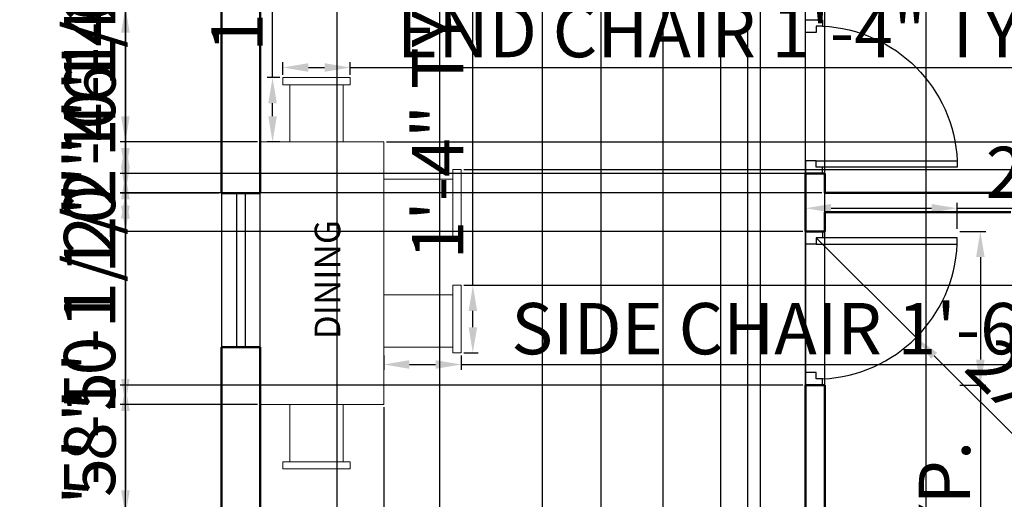
# Model space of a CAD drawing. Units: inches. Extents: x 1086 to 1501, y 383 to 973.
# Tile 3 of 7: x 1086 to 1316, y 611 to 723. Entities that reach past the tile are written whole.
import ezdxf

# ---------------------------------------------------------------- set-up
doc = ezdxf.new("R2010")
doc.units = ezdxf.units.IN
for name, color, linetype, lineweight in [('A-ANNO-DIMS', 2, 'Continuous', 18), ('A-AREA-IDEN', 7, 'Continuous', 25), ('door', 10, 'Continuous', 25), ('furniture', 255, 'Continuous', 18), ('wall', 7, 'Continuous', 50), ('window', 81, 'Continuous', 25)]:
    doc.layers.add(name, color=color, linetype=linetype, lineweight=lineweight)
doc.styles.get("Standard").update_dxf_attribs({"font": 'arial.ttf'})
doc.dimstyles.new('ISO-25', dxfattribs={"dimtxt": 12, "dimasz": 6, "dimexe": 1.25, "dimexo": 0.625, "dimtad": 1, "dimdec": 1, "dimlunit": 3, "dimtxsty": 'Standard', "dimcen": 2.5, "dimadec": 0, "dimazin": 0, "dimtfac": 1, "dimtdec": 1, "dimtmove": 0, "dimatfit": 3, "dimfxl": 1, "dimarcsym": 0})

# ---------------------------------------------------------------- blocks, each defined once
blk = doc.blocks.new('d2')
at = {"layer": 'door'}
blk.add_line((1603.89, 600.63), (1639.89, 600.63), dxfattribs=at)
blk.add_lwpolyline([(1605.39, 603.13), (1606.89, 603.13), (1606.89, 636.13), (1605.39, 636.13)], close=True, dxfattribs=at)
for points in [[(1606.89, 600.63), (1603.89, 600.63), (1603.89, 604.63), (1605.39, 604.63), (1605.39, 603.13), (1606.89, 603.13), (1606.89, 600.63)], [(1636.89, 600.63), (1639.89, 600.63), (1639.89, 604.63), (1638.39, 604.63), (1638.39, 603.13), (1636.89, 603.13), (1636.89, 600.63)]]:
    blk.add_lwpolyline(points, dxfattribs=at)
blk.add_arc((1605.39, 603.13), 33.03, 2.6026, 87.3974, dxfattribs=at)
blk = doc.blocks.new('w1')
at = {"layer": 'window'}
for p, q in [((1475.33, 845.32), (1475.33, 809.32)), ((1477.33, 845.32), (1477.33, 809.32))]:
    blk.add_line(p, q, dxfattribs=at)
blk.add_lwpolyline([(1471.83, 809.32), (1480.83, 809.32), (1480.83, 845.32), (1471.83, 845.32)], close=True, dxfattribs=at)
blk = doc.blocks.new('CHAIR-DINING-END')
for points in [[(0, 13.37), (15.81, 13.37), (15.81, 15.03), (0, 15.03)], [(1.64, 0), (14.11, 0), (14.11, 13.37), (1.64, 13.37)]]:
    blk.add_lwpolyline(points, close=True)
blk = doc.blocks.new('CHAIR-DINING-SIDE')
for points in [[(16.15, 15.81), (18.13, 15.81), (18.13, 0), (16.15, 0)], [(0, 13.58), (16.15, 13.58), (16.15, 1.34), (0, 1.34)]]:
    blk.add_lwpolyline(points, close=True)
blk = doc.blocks.new('*D19')
at = {"layer": 'A-ANNO-DIMS', "color": 0, "lineweight": -2, "transparency": 16777216}
for p, q in [((1306.05, 673.21), (1312.08, 673.21)), ((1310.83, 667.21), (1310.83, 643.21)), ((1306.05, 637.21), (1312.08, 637.21)), ((1310.83, 637.21), (1310.83, 411.12))]:
    blk.add_line(p, q, dxfattribs=at)
at = {"layer": 'A-ANNO-DIMS', "color": 0, "transparency": 16777216}
for points in [[(1309.83, 667.21), (1311.83, 667.21), (1310.83, 673.21)], [(1309.83, 643.21), (1311.83, 643.21), (1310.83, 637.21)]]:
    blk.add_solid(points, dxfattribs=at)
at = {"layer": 'Defpoints', "color": 0, "transparency": 16777216}
for p in [(1305.43, 673.21), (1305.43, 637.21), (1310.83, 637.21)]:
    blk.add_point(p, dxfattribs=at)
at = {"layer": 'A-ANNO-DIMS', "color": 0, "transparency": 16777216, "insert": (1303.99, 521.16), "char_height": 12, "attachment_point": 5, "rotation": 90}
blk.add_mtext('BEDROOM DOOR 3\'-0" TYP.', dxfattribs=at)
blk = doc.blocks.new('*D20')
at = {"layer": 'A-ANNO-DIMS', "color": 0, "lineweight": -2, "transparency": 16777216}
for p, q in [((1269.93, 673.83), (1269.93, 679.86)), ((1305.43, 673.83), (1305.43, 679.86)), ((1275.93, 678.61), (1299.43, 678.61)), ((1305.43, 678.61), (1423.32, 678.61))]:
    blk.add_line(p, q, dxfattribs=at)
at = {"layer": 'A-ANNO-DIMS', "color": 0, "transparency": 16777216}
for points in [[(1275.93, 679.61), (1275.93, 677.61), (1269.93, 678.61)], [(1299.43, 679.61), (1299.43, 677.61), (1305.43, 678.61)]]:
    blk.add_solid(points, dxfattribs=at)
at = {"layer": 'Defpoints', "color": 0, "transparency": 16777216}
for p in [(1305.43, 678.61), (1269.93, 673.21), (1305.43, 673.21)]:
    blk.add_point(p, dxfattribs=at)
at = {"layer": 'A-ANNO-DIMS', "color": 0, "transparency": 16777216, "insert": (1367.37, 685.44), "char_height": 12, "attachment_point": 5}
blk.add_mtext('2\'-11 1/2" TYP.', dxfattribs=at)
blk = doc.blocks.new('*D25')
at = {"layer": 'A-ANNO-DIMS', "color": 0, "lineweight": -2, "transparency": 16777216}
for p, q in [((1147.7, 709.78), (1147.7, 712.78)), ((1153.7, 711.53), (1157.51, 711.53)), ((1163.51, 709.78), (1163.51, 712.78)), ((1163.51, 711.53), (1340.15, 711.53))]:
    blk.add_line(p, q, dxfattribs=at)
at = {"layer": 'A-ANNO-DIMS', "color": 0, "transparency": 16777216}
for points in [[(1153.7, 712.53), (1153.7, 710.53), (1147.7, 711.53)], [(1157.51, 712.53), (1157.51, 710.53), (1163.51, 711.53)]]:
    blk.add_solid(points, dxfattribs=at)
at = {"layer": 'Defpoints', "color": 0, "transparency": 16777216}
for p in [(1163.51, 711.53), (1147.7, 709.16), (1163.51, 709.16)]:
    blk.add_point(p, dxfattribs=at)
at = {"layer": 'A-ANNO-DIMS', "color": 0, "transparency": 16777216, "insert": (1254.83, 718.36), "char_height": 12, "attachment_point": 5}
blk.add_mtext('END CHAIR 1\'-4" TYP.', dxfattribs=at)
blk = doc.blocks.new('*D26')
at = {"layer": 'A-ANNO-DIMS', "color": 0, "lineweight": -2, "transparency": 16777216}
for p, q in [((1145.33, 709.16), (1145.33, 788.42)), ((1147.07, 709.16), (1144.08, 709.16)), ((1145.33, 700.13), (1145.33, 703.16)), ((1147.07, 694.13), (1144.08, 694.13))]:
    blk.add_line(p, q, dxfattribs=at)
at = {"layer": 'A-ANNO-DIMS', "color": 0, "transparency": 16777216}
for points in [[(1144.33, 703.16), (1146.33, 703.16), (1145.33, 709.16)], [(1144.33, 700.13), (1146.33, 700.13), (1145.33, 694.13)]]:
    blk.add_solid(points, dxfattribs=at)
at = {"layer": 'Defpoints', "color": 0, "transparency": 16777216}
for p in [(1145.33, 709.16), (1147.7, 709.16), (1147.7, 694.13)]:
    blk.add_point(p, dxfattribs=at)
at = {"layer": 'A-ANNO-DIMS', "color": 0, "transparency": 16777216, "insert": (1138.57, 751.79), "char_height": 12, "attachment_point": 5, "rotation": 90}
blk.add_mtext('1\'-3" TYP.', dxfattribs=at)
blk = doc.blocks.new('*D27')
at = {"layer": 'A-ANNO-DIMS', "color": 0, "lineweight": -2, "transparency": 16777216}
for p, q in [((1171.32, 644.17), (1171.32, 640.82)), ((1189.45, 644.17), (1189.45, 640.82)), ((1177.32, 642.07), (1183.45, 642.07)), ((1189.45, 642.07), (1370.39, 642.07))]:
    blk.add_line(p, q, dxfattribs=at)
at = {"layer": 'A-ANNO-DIMS', "color": 0, "transparency": 16777216}
for points in [[(1177.32, 643.07), (1177.32, 641.07), (1171.32, 642.07)], [(1183.45, 643.07), (1183.45, 641.07), (1189.45, 642.07)]]:
    blk.add_solid(points, dxfattribs=at)
at = {"layer": 'Defpoints', "color": 0, "transparency": 16777216}
for p in [(1171.32, 644.79), (1189.45, 644.79), (1189.45, 642.07)]:
    blk.add_point(p, dxfattribs=at)
at = {"layer": 'A-ANNO-DIMS', "color": 0, "transparency": 16777216, "insert": (1282.92, 648.9), "char_height": 12, "attachment_point": 5}
blk.add_mtext('SIDE CHAIR 1\'-6" TYP.', dxfattribs=at)
blk = doc.blocks.new('*D28')
at = {"layer": 'A-ANNO-DIMS', "color": 0, "lineweight": -2, "transparency": 16777216}
for p, q in [((1192.17, 660.6), (1192.17, 739.87)), ((1190.08, 660.6), (1193.42, 660.6)), ((1192.17, 650.79), (1192.17, 654.6)), ((1190.08, 644.79), (1193.42, 644.79))]:
    blk.add_line(p, q, dxfattribs=at)
at = {"layer": 'A-ANNO-DIMS', "color": 0, "transparency": 16777216}
for points in [[(1191.17, 654.6), (1193.17, 654.6), (1192.17, 660.6)], [(1191.17, 650.79), (1193.17, 650.79), (1192.17, 644.79)]]:
    blk.add_solid(points, dxfattribs=at)
at = {"layer": 'Defpoints', "color": 0, "transparency": 16777216}
for p in [(1189.45, 660.6), (1192.17, 660.6), (1189.45, 644.79)]:
    blk.add_point(p, dxfattribs=at)
at = {"layer": 'A-ANNO-DIMS', "color": 0, "transparency": 16777216, "insert": (1185.52, 703.24), "char_height": 12, "attachment_point": 5, "rotation": 90}
blk.add_mtext('1\'-4" TYP.', dxfattribs=at)
blk = doc.blocks.new('*D33')
at = {"layer": 'A-ANNO-DIMS', "color": 0, "lineweight": -2, "transparency": 16777216}
for p, q in [((1132.8, 760.21), (1109.68, 760.21)), ((1110.93, 754.21), (1110.93, 688.12)), ((1132.8, 682.12), (1109.68, 682.12))]:
    blk.add_line(p, q, dxfattribs=at)
at = {"layer": 'A-ANNO-DIMS', "color": 0, "transparency": 16777216}
for points in [[(1109.93, 754.21), (1111.93, 754.21), (1110.93, 760.21)], [(1109.93, 688.12), (1111.93, 688.12), (1110.93, 682.12)]]:
    blk.add_solid(points, dxfattribs=at)
at = {"layer": 'Defpoints', "color": 0, "transparency": 16777216}
for p in [(1133.43, 760.21), (1110.93, 682.12), (1133.43, 682.12)]:
    blk.add_point(p, dxfattribs=at)
at = {"layer": 'A-ANNO-DIMS', "color": 0, "transparency": 16777216, "insert": (1104.18, 721.16), "char_height": 12, "attachment_point": 5, "rotation": 90}
blk.add_mtext('6\'-6"', dxfattribs=at)
blk = doc.blocks.new('*D40')
at = {"layer": 'A-ANNO-DIMS', "color": 0, "lineweight": -2, "transparency": 16777216}
for p, q in [((1142.43, 502.33), (1142.43, 867.19)), ((1148.43, 865.94), (1263.93, 865.94)), ((1269.93, 502.33), (1269.93, 867.19))]:
    blk.add_line(p, q, dxfattribs=at)
at = {"layer": 'A-ANNO-DIMS', "color": 0, "transparency": 16777216}
for points in [[(1148.43, 866.94), (1148.43, 864.94), (1142.43, 865.94)], [(1263.93, 866.94), (1263.93, 864.94), (1269.93, 865.94)]]:
    blk.add_solid(points, dxfattribs=at)
at = {"layer": 'Defpoints', "color": 0, "transparency": 16777216}
for p in [(1269.93, 865.94), (1142.43, 501.71), (1269.93, 501.71)]:
    blk.add_point(p, dxfattribs=at)
at = {"layer": 'A-ANNO-DIMS', "color": 0, "transparency": 16777216, "insert": (1206.18, 872.77), "char_height": 12, "attachment_point": 5}
blk.add_mtext('10\'-7 1/2"', dxfattribs=at)
blk = doc.blocks.new('*D41')
at = {"layer": 'A-ANNO-DIMS', "color": 0, "lineweight": -2, "transparency": 16777216}
for p, q in [((1141.8, 725.71), (1109.68, 725.71)), ((1110.93, 507.71), (1110.93, 719.71)), ((1141.8, 501.71), (1109.68, 501.71))]:
    blk.add_line(p, q, dxfattribs=at)
at = {"layer": 'A-ANNO-DIMS', "color": 0, "transparency": 16777216}
for points in [[(1109.93, 719.71), (1111.93, 719.71), (1110.93, 725.71)], [(1109.93, 507.71), (1111.93, 507.71), (1110.93, 501.71)]]:
    blk.add_solid(points, dxfattribs=at)
at = {"layer": 'Defpoints', "color": 0, "transparency": 16777216}
for p in [(1110.93, 725.71), (1142.43, 725.71), (1142.43, 501.71)]:
    blk.add_point(p, dxfattribs=at)
at = {"layer": 'A-ANNO-DIMS', "color": 0, "transparency": 16777216, "insert": (1104.18, 613.71), "char_height": 12, "attachment_point": 5, "rotation": 90}
blk.add_mtext('18\'-8"', dxfattribs=at)
blk = doc.blocks.new('*D42')
at = {"layer": 'A-ANNO-DIMS', "color": 0, "lineweight": -2, "transparency": 16777216}
for p, q in [((1256.43, 502.33), (1256.43, 867.19)), ((1262.43, 865.94), (1263.93, 865.94)), ((1269.93, 502.33), (1269.93, 867.19)), ((1269.93, 865.94), (1335.91, 865.94))]:
    blk.add_line(p, q, dxfattribs=at)
at = {"layer": 'A-ANNO-DIMS', "color": 0, "transparency": 16777216}
for points in [[(1262.43, 866.94), (1262.43, 864.94), (1256.43, 865.94)], [(1263.93, 866.94), (1263.93, 864.94), (1269.93, 865.94)]]:
    blk.add_solid(points, dxfattribs=at)
at = {"layer": 'Defpoints', "color": 0, "transparency": 16777216}
for p in [(1269.93, 865.94), (1256.43, 501.71), (1269.93, 501.71)]:
    blk.add_point(p, dxfattribs=at)
at = {"layer": 'A-ANNO-DIMS', "color": 0, "transparency": 16777216, "insert": (1305.92, 872.77), "char_height": 12, "attachment_point": 5}
blk.add_mtext('1\'-1 1/2"', dxfattribs=at)
blk = doc.blocks.new('*D43')
at = {"layer": 'A-ANNO-DIMS', "color": 0, "lineweight": -2, "transparency": 16777216}
for p, q in [((1208.43, 497.83), (1208.43, 867.19)), ((1214.43, 865.94), (1250.43, 865.94)), ((1256.43, 497.83), (1256.43, 867.19))]:
    blk.add_line(p, q, dxfattribs=at)
at = {"layer": 'A-ANNO-DIMS', "color": 0, "transparency": 16777216}
for points in [[(1214.43, 866.94), (1214.43, 864.94), (1208.43, 865.94)], [(1250.43, 866.94), (1250.43, 864.94), (1256.43, 865.94)]]:
    blk.add_solid(points, dxfattribs=at)
at = {"layer": 'Defpoints', "color": 0, "transparency": 16777216}
for p in [(1256.43, 865.94), (1208.43, 497.21), (1256.43, 497.21)]:
    blk.add_point(p, dxfattribs=at)
at = {"layer": 'A-ANNO-DIMS', "color": 0, "transparency": 16777216, "insert": (1232.43, 872.69), "char_height": 12, "attachment_point": 5}
blk.add_mtext('4\'-0"', dxfattribs=at)
blk = doc.blocks.new('*D45')
at = {"layer": 'A-ANNO-DIMS', "color": 0, "lineweight": -2, "transparency": 16777216}
for p, q in [((1259.43, 497.83), (1259.43, 867.19)), ((1265.43, 865.94), (1352.43, 865.94)), ((1358.43, 497.83), (1358.43, 867.19))]:
    blk.add_line(p, q, dxfattribs=at)
at = {"layer": 'A-ANNO-DIMS', "color": 0, "transparency": 16777216}
for points in [[(1265.43, 866.94), (1265.43, 864.94), (1259.43, 865.94)], [(1352.43, 866.94), (1352.43, 864.94), (1358.43, 865.94)]]:
    blk.add_solid(points, dxfattribs=at)
at = {"layer": 'Defpoints', "color": 0, "transparency": 16777216}
for p in [(1358.43, 865.94), (1259.43, 497.21), (1358.43, 497.21)]:
    blk.add_point(p, dxfattribs=at)
at = {"layer": 'A-ANNO-DIMS', "color": 0, "transparency": 16777216, "insert": (1308.93, 872.7), "char_height": 12, "attachment_point": 5}
blk.add_mtext('8\'-3"', dxfattribs=at)
blk = doc.blocks.new('*D49')
at = {"layer": 'A-ANNO-DIMS', "color": 0, "lineweight": -2, "transparency": 16777216}
for p, q in [((1110.93, 760.21), (1110.93, 766.21)), ((1218.3, 754.21), (1109.68, 754.21)), ((1110.93, 754.21), (1110.93, 749.71)), ((1218.3, 749.71), (1109.68, 749.71)), ((1110.93, 743.71), (1110.93, 676.6))]:
    blk.add_line(p, q, dxfattribs=at)
at = {"layer": 'A-ANNO-DIMS', "color": 0, "transparency": 16777216}
for points in [[(1109.93, 760.21), (1111.93, 760.21), (1110.93, 754.21)], [(1109.93, 743.71), (1111.93, 743.71), (1110.93, 749.71)]]:
    blk.add_solid(points, dxfattribs=at)
at = {"layer": 'Defpoints', "color": 0, "transparency": 16777216}
for p in [(1218.93, 754.21), (1110.93, 749.71), (1218.93, 749.71)]:
    blk.add_point(p, dxfattribs=at)
at = {"layer": 'A-ANNO-DIMS', "color": 0, "transparency": 16777216, "insert": (1104.1, 707.15), "char_height": 12, "attachment_point": 5, "rotation": 90}
blk.add_mtext('0\'-4 1/2"', dxfattribs=at)
blk = doc.blocks.new('*D50')
at = {"layer": 'A-ANNO-DIMS', "color": 0, "lineweight": -2, "transparency": 16777216}
for p, q in [((1184.43, 502.33), (1184.43, 867.19)), ((1190.43, 865.94), (1202.43, 865.94)), ((1208.43, 502.33), (1208.43, 867.19)), ((1208.43, 865.94), (1247.78, 865.94))]:
    blk.add_line(p, q, dxfattribs=at)
at = {"layer": 'A-ANNO-DIMS', "color": 0, "transparency": 16777216}
for points in [[(1190.43, 866.94), (1190.43, 864.94), (1184.43, 865.94)], [(1202.43, 866.94), (1202.43, 864.94), (1208.43, 865.94)]]:
    blk.add_solid(points, dxfattribs=at)
at = {"layer": 'Defpoints', "color": 0, "transparency": 16777216}
for p in [(1208.43, 865.94), (1184.43, 501.71), (1208.43, 501.71)]:
    blk.add_point(p, dxfattribs=at)
at = {"layer": 'A-ANNO-DIMS', "color": 0, "transparency": 16777216, "insert": (1231.11, 872.69), "char_height": 12, "attachment_point": 5}
blk.add_mtext('2\'-0"', dxfattribs=at)
blk = doc.blocks.new('*D52')
at = {"layer": 'A-ANNO-DIMS', "color": 0, "lineweight": -2, "transparency": 16777216}
for p, q in [((1110.93, 692.71), (1110.93, 759.82)), ((1273.8, 686.71), (1109.68, 686.71)), ((1110.93, 682.21), (1110.93, 686.71)), ((1273.8, 682.21), (1109.68, 682.21)), ((1110.93, 676.21), (1110.93, 670.21))]:
    blk.add_line(p, q, dxfattribs=at)
at = {"layer": 'A-ANNO-DIMS', "color": 0, "transparency": 16777216}
for points in [[(1109.93, 692.71), (1111.93, 692.71), (1110.93, 686.71)], [(1109.93, 676.21), (1111.93, 676.21), (1110.93, 682.21)]]:
    blk.add_solid(points, dxfattribs=at)
at = {"layer": 'Defpoints', "color": 0, "transparency": 16777216}
for p in [(1110.93, 686.71), (1274.43, 686.71), (1274.43, 682.21)]:
    blk.add_point(p, dxfattribs=at)
at = {"layer": 'A-ANNO-DIMS', "color": 0, "transparency": 16777216, "insert": (1104.1, 729.26), "char_height": 12, "attachment_point": 5, "rotation": 90}
blk.add_mtext('0\'-4 1/2"', dxfattribs=at)
blk = doc.blocks.new('*D53')
at = {"layer": 'A-ANNO-DIMS', "color": 0, "lineweight": -2, "transparency": 16777216}
for p, q in [((1110.93, 686.71), (1110.93, 752.69)), ((1269.3, 686.71), (1109.68, 686.71)), ((1110.93, 679.21), (1110.93, 680.71)), ((1269.3, 673.21), (1109.68, 673.21))]:
    blk.add_line(p, q, dxfattribs=at)
at = {"layer": 'A-ANNO-DIMS', "color": 0, "transparency": 16777216}
for points in [[(1109.93, 680.71), (1111.93, 680.71), (1110.93, 686.71)], [(1109.93, 679.21), (1111.93, 679.21), (1110.93, 673.21)]]:
    blk.add_solid(points, dxfattribs=at)
at = {"layer": 'Defpoints', "color": 0, "transparency": 16777216}
for p in [(1110.93, 686.71), (1269.93, 686.71), (1269.93, 673.21)]:
    blk.add_point(p, dxfattribs=at)
at = {"layer": 'A-ANNO-DIMS', "color": 0, "transparency": 16777216, "insert": (1104.1, 722.7), "char_height": 12, "attachment_point": 5, "rotation": 90}
blk.add_mtext('1\'-1 1/2"', dxfattribs=at)
blk = doc.blocks.new('*D58')
at = {"layer": 'A-ANNO-DIMS', "color": 0, "lineweight": -2, "transparency": 16777216}
for p, q in [((1250.08, 809.82), (1250.08, 392.46)), ((1222.08, 799.32), (1222.08, 392.46)), ((1228.08, 393.71), (1244.08, 393.71)), ((1250.08, 393.71), (1289.44, 393.71))]:
    blk.add_line(p, q, dxfattribs=at)
at = {"layer": 'A-ANNO-DIMS', "color": 0, "transparency": 16777216}
for points in [[(1228.08, 394.71), (1228.08, 392.71), (1222.08, 393.71)], [(1244.08, 394.71), (1244.08, 392.71), (1250.08, 393.71)]]:
    blk.add_solid(points, dxfattribs=at)
at = {"layer": 'Defpoints', "color": 0, "transparency": 16777216}
for p in [(1250.08, 810.44), (1222.08, 799.94), (1250.08, 393.71)]:
    blk.add_point(p, dxfattribs=at)
at = {"layer": 'A-ANNO-DIMS', "color": 0, "transparency": 16777216, "insert": (1272.76, 400.36), "char_height": 12, "attachment_point": 5}
blk.add_mtext('2\'-4"', dxfattribs=at)
blk = doc.blocks.new('*D60')
at = {"layer": 'A-ANNO-DIMS', "color": 0, "lineweight": -2, "transparency": 16777216}
for p, q in [((1322.43, 629.08), (1322.43, 392.46)), ((1326.93, 629.08), (1326.93, 392.46)), ((1316.43, 393.71), (1310.43, 393.71)), ((1322.43, 393.71), (1326.93, 393.71)), ((1332.93, 393.71), (1400.04, 393.71))]:
    blk.add_line(p, q, dxfattribs=at)
at = {"layer": 'A-ANNO-DIMS', "color": 0, "transparency": 16777216}
for points in [[(1316.43, 394.71), (1316.43, 392.71), (1322.43, 393.71)], [(1332.93, 394.71), (1332.93, 392.71), (1326.93, 393.71)]]:
    blk.add_solid(points, dxfattribs=at)
at = {"layer": 'Defpoints', "color": 0, "transparency": 16777216}
for p in [(1322.43, 629.71), (1326.93, 629.71), (1326.93, 393.71)]:
    blk.add_point(p, dxfattribs=at)
at = {"layer": 'A-ANNO-DIMS', "color": 0, "transparency": 16777216, "insert": (1369.49, 400.54), "char_height": 12, "attachment_point": 5}
blk.add_mtext('0\'-4 1/2"', dxfattribs=at)
blk = doc.blocks.new('*D61')
at = {"layer": 'A-ANNO-DIMS', "color": 0, "lineweight": -2, "transparency": 16777216}
for p, q in [((1376.11, 865.94), (1310.13, 865.94)), ((1382.11, 674.69), (1382.11, 867.19)), ((1394.43, 865.94), (1382.11, 865.94)), ((1394.43, 678.33), (1394.43, 867.19)), ((1400.43, 865.94), (1406.43, 865.94))]:
    blk.add_line(p, q, dxfattribs=at)
at = {"layer": 'A-ANNO-DIMS', "color": 0, "transparency": 16777216}
for points in [[(1376.11, 866.94), (1376.11, 864.94), (1382.11, 865.94)], [(1400.43, 866.94), (1400.43, 864.94), (1394.43, 865.94)]]:
    blk.add_solid(points, dxfattribs=at)
at = {"layer": 'Defpoints', "color": 0, "transparency": 16777216}
for p in [(1382.11, 865.94), (1394.43, 677.71), (1382.11, 674.06)]:
    blk.add_point(p, dxfattribs=at)
at = {"layer": 'A-ANNO-DIMS', "color": 0, "transparency": 16777216, "insert": (1340.12, 872.77), "char_height": 12, "attachment_point": 5}
blk.add_mtext('1\'-0 1/2"', dxfattribs=at)
blk = doc.blocks.new('*D63')
at = {"layer": 'A-ANNO-DIMS', "color": 0, "lineweight": -2, "transparency": 16777216}
for p, q in [((1142.43, 632.08), (1142.43, 392.46)), ((1171.32, 632.08), (1171.32, 392.46)), ((1148.43, 393.71), (1165.32, 393.71)), ((1171.32, 393.71), (1210.68, 393.71))]:
    blk.add_line(p, q, dxfattribs=at)
at = {"layer": 'A-ANNO-DIMS', "color": 0, "transparency": 16777216}
for points in [[(1148.43, 394.71), (1148.43, 392.71), (1142.43, 393.71)], [(1165.32, 394.71), (1165.32, 392.71), (1171.32, 393.71)]]:
    blk.add_solid(points, dxfattribs=at)
at = {"layer": 'Defpoints', "color": 0, "transparency": 16777216}
for p in [(1142.43, 632.71), (1171.32, 632.71), (1171.32, 393.71)]:
    blk.add_point(p, dxfattribs=at)
at = {"layer": 'A-ANNO-DIMS', "color": 0, "transparency": 16777216, "insert": (1194, 400.46), "char_height": 12, "attachment_point": 5}
blk.add_mtext('2\'-5"', dxfattribs=at)
blk = doc.blocks.new('*D64')
at = {"layer": 'A-ANNO-DIMS', "color": 0, "lineweight": -2, "transparency": 16777216}
for p, q in [((1141.8, 694.13), (1109.68, 694.13)), ((1110.93, 688.13), (1110.93, 638.71)), ((1141.8, 632.71), (1109.68, 632.71))]:
    blk.add_line(p, q, dxfattribs=at)
at = {"layer": 'A-ANNO-DIMS', "color": 0, "transparency": 16777216}
for points in [[(1109.93, 688.13), (1111.93, 688.13), (1110.93, 694.13)], [(1109.93, 638.71), (1111.93, 638.71), (1110.93, 632.71)]]:
    blk.add_solid(points, dxfattribs=at)
at = {"layer": 'Defpoints', "color": 0, "transparency": 16777216}
for p in [(1142.43, 694.13), (1110.93, 632.71), (1142.43, 632.71)]:
    blk.add_point(p, dxfattribs=at)
at = {"layer": 'A-ANNO-DIMS', "color": 0, "transparency": 16777216, "insert": (1104.1, 663.42), "char_height": 12, "attachment_point": 5, "rotation": 90}
blk.add_mtext('5\'-1 1/2"', dxfattribs=at)
blk = doc.blocks.new('*D65')
at = {"layer": 'A-ANNO-DIMS', "color": 0, "lineweight": -2, "transparency": 16777216}
for p, q in [((1110.93, 725.71), (1110.93, 793.02)), ((1141.8, 725.71), (1109.68, 725.71)), ((1110.93, 700.13), (1110.93, 719.71)), ((1141.8, 694.13), (1109.68, 694.13))]:
    blk.add_line(p, q, dxfattribs=at)
at = {"layer": 'A-ANNO-DIMS', "color": 0, "transparency": 16777216}
for points in [[(1109.93, 719.71), (1111.93, 719.71), (1110.93, 725.71)], [(1109.93, 700.13), (1111.93, 700.13), (1110.93, 694.13)]]:
    blk.add_solid(points, dxfattribs=at)
at = {"layer": 'Defpoints', "color": 0, "transparency": 16777216}
for p in [(1110.93, 725.71), (1142.43, 725.71), (1142.43, 694.13)]:
    blk.add_point(p, dxfattribs=at)
at = {"layer": 'A-ANNO-DIMS', "color": 0, "transparency": 16777216, "insert": (1104.1, 762.36), "char_height": 12, "attachment_point": 5, "rotation": 90}
blk.add_mtext('2\'-7 1/2"', dxfattribs=at)
blk = doc.blocks.new('*D66')
at = {"layer": 'A-ANNO-DIMS', "color": 0, "lineweight": -2, "transparency": 16777216}
for p, q in [((1190.08, 687.66), (1428.36, 687.66)), ((1427.11, 681.66), (1427.11, 666.6)), ((1190.08, 660.6), (1428.36, 660.6)), ((1427.11, 660.6), (1427.11, 621.25))]:
    blk.add_line(p, q, dxfattribs=at)
at = {"layer": 'A-ANNO-DIMS', "color": 0, "transparency": 16777216}
for points in [[(1426.11, 681.66), (1428.11, 681.66), (1427.11, 687.66)], [(1426.11, 666.6), (1428.11, 666.6), (1427.11, 660.6)]]:
    blk.add_solid(points, dxfattribs=at)
at = {"layer": 'Defpoints', "color": 0, "transparency": 16777216}
for p in [(1189.45, 687.66), (1189.45, 660.6), (1427.11, 660.6)]:
    blk.add_point(p, dxfattribs=at)
at = {"layer": 'A-ANNO-DIMS', "color": 0, "transparency": 16777216, "insert": (1420.36, 637.93), "char_height": 12, "attachment_point": 5, "rotation": 90}
blk.add_mtext('2\'-3"', dxfattribs=at)
blk = doc.blocks.new('*D67')
at = {"layer": 'A-ANNO-DIMS', "color": 0, "lineweight": -2, "transparency": 16777216}
for p, q in [((1427.11, 700.13), (1427.11, 706.13)), ((1171.95, 694.13), (1428.36, 694.13)), ((1427.11, 694.13), (1427.11, 687.66)), ((1190.08, 687.66), (1428.36, 687.66)), ((1427.11, 681.66), (1427.11, 614.55))]:
    blk.add_line(p, q, dxfattribs=at)
at = {"layer": 'A-ANNO-DIMS', "color": 0, "transparency": 16777216}
for points in [[(1426.11, 700.13), (1428.11, 700.13), (1427.11, 694.13)], [(1426.11, 681.66), (1428.11, 681.66), (1427.11, 687.66)]]:
    blk.add_solid(points, dxfattribs=at)
at = {"layer": 'Defpoints', "color": 0, "transparency": 16777216}
for p in [(1171.32, 694.13), (1189.45, 687.66), (1427.11, 687.66)]:
    blk.add_point(p, dxfattribs=at)
at = {"layer": 'A-ANNO-DIMS', "color": 0, "transparency": 16777216, "insert": (1420.28, 645.1), "char_height": 12, "attachment_point": 5, "rotation": 90}
blk.add_mtext('0\'-6 1/2"', dxfattribs=at)
blk = doc.blocks.new('*D68')
at = {"layer": 'A-ANNO-DIMS', "color": 0, "lineweight": -2, "transparency": 16777216}
for p, q in [((1110.93, 606.65), (1110.93, 683.08)), ((1262.93, 606.65), (1109.68, 606.65)), ((1110.93, 542.31), (1110.93, 600.65)), ((1262.93, 536.31), (1109.68, 536.31))]:
    blk.add_line(p, q, dxfattribs=at)
at = {"layer": 'A-ANNO-DIMS', "color": 0, "transparency": 16777216}
for points in [[(1109.93, 600.65), (1111.93, 600.65), (1110.93, 606.65)], [(1109.93, 542.31), (1111.93, 542.31), (1110.93, 536.31)]]:
    blk.add_solid(points, dxfattribs=at)
at = {"layer": 'Defpoints', "color": 0, "transparency": 16777216}
for p in [(1110.93, 606.65), (1263.55, 606.65), (1263.55, 536.31)]:
    blk.add_point(p, dxfattribs=at)
at = {"layer": 'A-ANNO-DIMS', "color": 0, "transparency": 16777216, "insert": (1104.1, 647.86), "char_height": 12, "attachment_point": 5, "rotation": 90}
blk.add_mtext('5\'-10 1/2"', dxfattribs=at)
blk = doc.blocks.new('*D69')
at = {"layer": 'A-ANNO-DIMS', "color": 0, "lineweight": -2, "transparency": 16777216}
for p, q in [((1236.63, 603.21), (1236.63, 867.19)), ((1242.63, 865.94), (1263.93, 865.94)), ((1269.93, 603.25), (1269.93, 867.19)), ((1269.93, 865.94), (1337.25, 865.94))]:
    blk.add_line(p, q, dxfattribs=at)
at = {"layer": 'A-ANNO-DIMS', "color": 0, "transparency": 16777216}
for points in [[(1242.63, 866.94), (1242.63, 864.94), (1236.63, 865.94)], [(1263.93, 866.94), (1263.93, 864.94), (1269.93, 865.94)]]:
    blk.add_solid(points, dxfattribs=at)
at = {"layer": 'Defpoints', "color": 0, "transparency": 16777216}
for p in [(1269.93, 865.94), (1236.63, 602.59), (1269.93, 602.62)]:
    blk.add_point(p, dxfattribs=at)
at = {"layer": 'A-ANNO-DIMS', "color": 0, "transparency": 16777216, "insert": (1306.59, 872.77), "char_height": 12, "attachment_point": 5}
blk.add_mtext('2\'-9 1/2"', dxfattribs=at)
blk = doc.blocks.new('*D70')
at = {"layer": 'A-ANNO-DIMS', "color": 0, "lineweight": -2, "transparency": 16777216}
for p, q in [((1269.3, 637.21), (1109.68, 637.21)), ((1110.93, 631.21), (1110.93, 612.65)), ((1262.93, 606.65), (1109.68, 606.65)), ((1110.93, 606.65), (1110.93, 539.33))]:
    blk.add_line(p, q, dxfattribs=at)
at = {"layer": 'A-ANNO-DIMS', "color": 0, "transparency": 16777216}
for points in [[(1109.93, 631.21), (1111.93, 631.21), (1110.93, 637.21)], [(1109.93, 612.65), (1111.93, 612.65), (1110.93, 606.65)]]:
    blk.add_solid(points, dxfattribs=at)
at = {"layer": 'Defpoints', "color": 0, "transparency": 16777216}
for p in [(1269.93, 637.21), (1110.93, 606.65), (1263.55, 606.65)]:
    blk.add_point(p, dxfattribs=at)
at = {"layer": 'A-ANNO-DIMS', "color": 0, "transparency": 16777216, "insert": (1104.1, 569.99), "char_height": 12, "attachment_point": 5, "rotation": 90}
blk.add_mtext('2\'-6 1/2"', dxfattribs=at)
blk = doc.blocks.new('*D71')
at = {"layer": 'A-ANNO-DIMS', "color": 0, "lineweight": -2, "transparency": 16777216}
for p, q in [((1142.43, 589.29), (1142.43, 867.19)), ((1148.43, 865.94), (1154.43, 865.94)), ((1160.43, 589.29), (1160.43, 867.19)), ((1160.43, 865.94), (1198.45, 865.94))]:
    blk.add_line(p, q, dxfattribs=at)
at = {"layer": 'A-ANNO-DIMS', "color": 0, "transparency": 16777216}
for points in [[(1148.43, 866.94), (1148.43, 864.94), (1142.43, 865.94)], [(1154.43, 866.94), (1154.43, 864.94), (1160.43, 865.94)]]:
    blk.add_solid(points, dxfattribs=at)
at = {"layer": 'Defpoints', "color": 0, "transparency": 16777216}
for p in [(1160.43, 865.94), (1142.43, 588.67), (1160.43, 588.67)]:
    blk.add_point(p, dxfattribs=at)
at = {"layer": 'A-ANNO-DIMS', "color": 0, "transparency": 16777216, "insert": (1182.44, 872.69), "char_height": 12, "attachment_point": 5}
blk.add_mtext('1\'-6"', dxfattribs=at)
blk = doc.blocks.new('*D75')
at = {"layer": 'A-ANNO-DIMS', "color": 0, "lineweight": -2, "transparency": 16777216}
for p, q in [((1274.43, 723.33), (1274.43, 867.19)), ((1280.43, 865.94), (1304.55, 865.94)), ((1310.55, 724.51), (1310.55, 867.19))]:
    blk.add_line(p, q, dxfattribs=at)
at = {"layer": 'A-ANNO-DIMS', "color": 0, "transparency": 16777216}
for points in [[(1280.43, 866.94), (1280.43, 864.94), (1274.43, 865.94)], [(1304.55, 866.94), (1304.55, 864.94), (1310.55, 865.94)]]:
    blk.add_solid(points, dxfattribs=at)
at = {"layer": 'Defpoints', "color": 0, "transparency": 16777216}
for p in [(1310.55, 865.94), (1310.55, 723.89), (1274.43, 722.71)]:
    blk.add_point(p, dxfattribs=at)
at = {"layer": 'A-ANNO-DIMS', "color": 0, "transparency": 16777216, "insert": (1292.49, 872.7), "char_height": 12, "attachment_point": 5}
blk.add_mtext('3\'-0"', dxfattribs=at)
blk = doc.blocks.new('*D77')
at = {"layer": 'A-ANNO-DIMS', "color": 0, "lineweight": -2, "transparency": 16777216}
for p, q in [((1274.43, 502.33), (1274.43, 867.19)), ((1280.43, 865.94), (1292.14, 865.94)), ((1298.14, 513.04), (1298.14, 867.19)), ((1298.14, 865.94), (1373.44, 865.94))]:
    blk.add_line(p, q, dxfattribs=at)
at = {"layer": 'A-ANNO-DIMS', "color": 0, "transparency": 16777216}
for points in [[(1280.43, 866.94), (1280.43, 864.94), (1274.43, 865.94)], [(1292.14, 866.94), (1292.14, 864.94), (1298.14, 865.94)]]:
    blk.add_solid(points, dxfattribs=at)
at = {"layer": 'Defpoints', "color": 0, "transparency": 16777216}
for p in [(1298.14, 865.94), (1298.14, 512.42), (1274.43, 501.71)]:
    blk.add_point(p, dxfattribs=at)
at = {"layer": 'A-ANNO-DIMS', "color": 0, "transparency": 16777216, "insert": (1338.79, 872.77), "char_height": 12, "attachment_point": 5}
blk.add_mtext('1\'-11 1/2"', dxfattribs=at)
blk = doc.blocks.new('*D78')
at = {"layer": 'A-ANNO-DIMS', "color": 0, "lineweight": -2, "transparency": 16777216}
for p, q in [((1272.43, 671.71), (1295.79, 648.35)), ((1354.21, 589.92), (1300.03, 644.11))]:
    blk.add_line(p, q, dxfattribs=at)
at = {"layer": 'A-ANNO-DIMS', "color": 0, "transparency": 16777216}
blk.add_solid([(1300.74, 644.81), (1299.32, 643.4), (1295.79, 648.35)], dxfattribs=at)
at = {"layer": 'Defpoints', "color": 0, "transparency": 16777216}
for p in [(1272.43, 671.71), (1295.79, 648.35)]:
    blk.add_point(p, dxfattribs=at)
at = {"layer": 'A-ANNO-DIMS', "color": 0, "transparency": 16777216, "insert": (1334.02, 619.67), "char_height": 12, "attachment_point": 5, "rotation": 314.9994}
blk.add_mtext('2X R2\'-9"', dxfattribs=at)

msp = doc.modelspace()

# ---------------------------------------------------------------- linework, layer by layer
at = {"layer": 'furniture'}
msp.add_lwpolyline([(1142.43, 694.13), (1171.32, 694.13), (1171.32, 632.71), (1142.43, 632.71)], close=True, dxfattribs=at)
at = {"layer": 'wall'}
for p, q in [((1133.43, 760.21), (1133.43, 682.12)), ((1142.43, 725.71), (1142.43, 682.12)), ((1269.93, 673.21), (1269.93, 686.71)), ((1274.43, 686.71), (1269.93, 686.71)), ((1274.43, 682.21), (1274.43, 686.71)), ((1142.43, 682.12), (1133.43, 682.12)), ((1394.43, 682.21), (1274.43, 682.21)), ((1317.93, 677.71), (1274.43, 677.71)), ((1274.43, 673.21), (1274.43, 677.71)), ((1274.43, 673.21), (1269.93, 673.21)), ((1142.43, 646.12), (1133.43, 646.12)), ((1133.43, 646.12), (1133.43, 416.21)), ((1142.43, 646.12), (1142.43, 501.71)), ((1269.93, 501.71), (1269.93, 637.21)), ((1274.43, 637.21), (1269.93, 637.21)), ((1274.43, 501.71), (1274.43, 637.21))]:
    msp.add_line(p, q, dxfattribs=at)

# ---------------------------------------------------------------- block references
at = {"layer": 'door', "xscale": -1, "rotation": 270}
msp.add_blockref('d2', (669.3, -917.19), dxfattribs=at)
at = {"layer": 'door', "rotation": 270}
msp.add_blockref('d2', (669.3, 2277.1), dxfattribs=at)
at = {"layer": 'furniture'}
for name, p in [('CHAIR-DINING-END', (1147.7, 694.13)), ('CHAIR-DINING-SIDE', (1171.32, 671.85)), ('CHAIR-DINING-SIDE', (1171.32, 644.79))]:
    msp.add_blockref(name, p, dxfattribs=at)
at = {"layer": 'furniture', "extrusion": (0, 0, -1), "zscale": -1, "rotation": 180}
msp.add_blockref('CHAIR-DINING-END', (-1147.7, 632.71), dxfattribs=at)
at = {"layer": 'window'}
msp.add_blockref('w1', (-338.4, -163.2), dxfattribs=at)

# ---------------------------------------------------------------- texts
at = {"layer": 'A-AREA-IDEN', "insert": (1155.17, 646.12), "char_height": 6, "attachment_point": 1, "rotation": 90}
msp.add_mtext_dynamic_manual_height_columns(' DINING', width=53.2651, gutter_width=12.5, heights=[0], dxfattribs=at)

# ---------------------------------------------------------------- dimensions: what is measured, and where the dimension line sits
at = {"layer": 'A-ANNO-DIMS'}
for base, p1, p2, picture, middle in [((1269.93, 865.94), (1142.43, 501.71), (1269.93, 501.71), '*D40', (1206.18, 872.77)), ((1269.93, 865.94), (1236.63, 602.59), (1269.93, 602.62), '*D69', (1306.59, 872.77)), ((1269.93, 865.94), (1256.43, 501.71), (1269.93, 501.71), '*D42', (1305.92, 872.77)), ((1298.14, 865.94), (1274.43, 501.71), (1298.14, 512.42), '*D77', (1338.79, 872.77)), ((1382.11, 865.94), (1394.43, 677.71), (1382.11, 674.06), '*D61', (1340.12, 872.77)), ((1160.43, 865.94), (1142.43, 588.67), (1160.43, 588.67), '*D71', (1182.44, 872.69)), ((1208.43, 865.94), (1184.43, 501.71), (1208.43, 501.71), '*D50', (1231.11, 872.69)), ((1256.43, 865.94), (1208.43, 497.21), (1256.43, 497.21), '*D43', (1232.43, 872.69)), ((1358.43, 865.94), (1259.43, 497.21), (1358.43, 497.21), '*D45', (1308.93, 872.7)), ((1310.55, 865.94), (1274.43, 722.71), (1310.55, 723.89), '*D75', (1292.49, 872.7)), ((1250.08, 393.71), (1222.08, 799.94), (1250.08, 810.44), '*D58', (1272.76, 400.36)), ((1171.32, 393.71), (1142.43, 632.71), (1171.32, 632.71), '*D63', (1194, 400.46)), ((1326.93, 393.71), (1322.43, 629.71), (1326.93, 629.71), '*D60', (1369.49, 400.54))]:
    dim = msp.add_linear_dim(base=base, p1=p1, p2=p2, dimstyle='ISO-25', override={"dimdec": 1, "dimlfac": 1, "dimrnd": 0, "dimzin": 1, "dimdsep": 46, "dimlunit": 4, "dimfrac": 2}, dxfattribs=at)
    dim.commit()
    dim.dimension.update_dxf_attribs({"geometry": picture, "text_midpoint": middle})
for base, p1, p2, picture, middle in [((1110.93, 725.71), (1142.43, 694.13), (1142.43, 725.71), '*D65', (1104.1, 762.36)), ((1110.93, 749.71), (1218.93, 754.21), (1218.93, 749.71), '*D49', (1104.1, 707.15)), ((1110.93, 686.71), (1274.43, 682.21), (1274.43, 686.71), '*D52', (1104.1, 729.26)), ((1110.93, 682.12), (1133.43, 760.21), (1133.43, 682.12), '*D33', (1104.18, 721.16)), ((1110.93, 686.71), (1269.93, 673.21), (1269.93, 686.71), '*D53', (1104.1, 722.7)), ((1110.93, 725.71), (1142.43, 501.71), (1142.43, 725.71), '*D41', (1104.18, 613.71)), ((1427.11, 687.66), (1171.32, 694.13), (1189.45, 687.66), '*D67', (1420.28, 645.1)), ((1110.93, 632.71), (1142.43, 694.13), (1142.43, 632.71), '*D64', (1104.1, 663.42)), ((1427.11, 660.6), (1189.45, 687.66), (1189.45, 660.6), '*D66', (1420.36, 637.93)), ((1110.93, 606.65), (1263.55, 536.31), (1263.55, 606.65), '*D68', (1104.1, 647.86)), ((1110.93, 606.65), (1269.93, 637.21), (1263.55, 606.65), '*D70', (1104.1, 569.99))]:
    dim = msp.add_linear_dim(base=base, p1=p1, p2=p2, angle=90, dimstyle='ISO-25', override={"dimdec": 1, "dimlfac": 1, "dimrnd": 0, "dimzin": 1, "dimdsep": 46, "dimlunit": 4, "dimfrac": 2}, dxfattribs=at)
    dim.commit()
    dim.dimension.update_dxf_attribs({"geometry": picture, "text_midpoint": middle})
for base, p1, p2, angle, text, picture, middle in [((1145.33, 709.16), (1147.7, 694.13), (1147.7, 709.16), 90, '<> TYP.', '*D26', (1138.57, 751.79)), ((1192.17, 660.6), (1189.45, 644.79), (1189.45, 660.6), 90, '<> TYP.', '*D28', (1185.52, 703.24)), ((1310.83, 637.21), (1305.43, 673.21), (1305.43, 637.21), 270, 'BEDROOM DOOR <> TYP.', '*D19', (1303.99, 521.16))]:
    dim = msp.add_linear_dim(base=base, p1=p1, p2=p2, angle=angle, text=text, dimstyle='ISO-25', override={"dimdec": 1, "dimlfac": 1, "dimrnd": 0, "dimzin": 1, "dimdsep": 46, "dimlunit": 4, "dimfrac": 2}, dxfattribs=at)
    dim.commit()
    dim.dimension.update_dxf_attribs({"geometry": picture, "text_midpoint": middle})
for base, p1, p2, text, picture, middle in [((1163.51, 711.53), (1147.7, 709.16), (1163.51, 709.16), 'END CHAIR <> TYP.', '*D25', (1254.83, 718.36)), ((1305.43, 678.61), (1269.93, 673.21), (1305.43, 673.21), '<> TYP.', '*D20', (1367.37, 685.44)), ((1189.45, 642.07), (1171.32, 644.79), (1189.45, 644.79), 'SIDE CHAIR <> TYP.', '*D27', (1282.92, 648.9))]:
    dim = msp.add_linear_dim(base=base, p1=p1, p2=p2, text=text, dimstyle='ISO-25', override={"dimdec": 1, "dimlfac": 1, "dimrnd": 0, "dimzin": 1, "dimdsep": 46, "dimlunit": 4, "dimfrac": 2}, dxfattribs=at)
    dim.commit()
    dim.dimension.update_dxf_attribs({"geometry": picture, "text_midpoint": middle})
dim = msp.add_radius_dim(center=(1272.43, 671.71), mpoint=(1295.79, 648.35), text='2X <>', dimstyle='ISO-25', override={"dimdec": 1, "dimlfac": 1, "dimrnd": 0, "dimzin": 1, "dimdsep": 46, "dimlunit": 4, "dimfrac": 2}, dxfattribs=at)
dim.commit()
dim.dimension.update_dxf_attribs({"geometry": '*D78', "text_midpoint": (1334.02, 619.67)})

doc.saveas('drawing.dxf')
